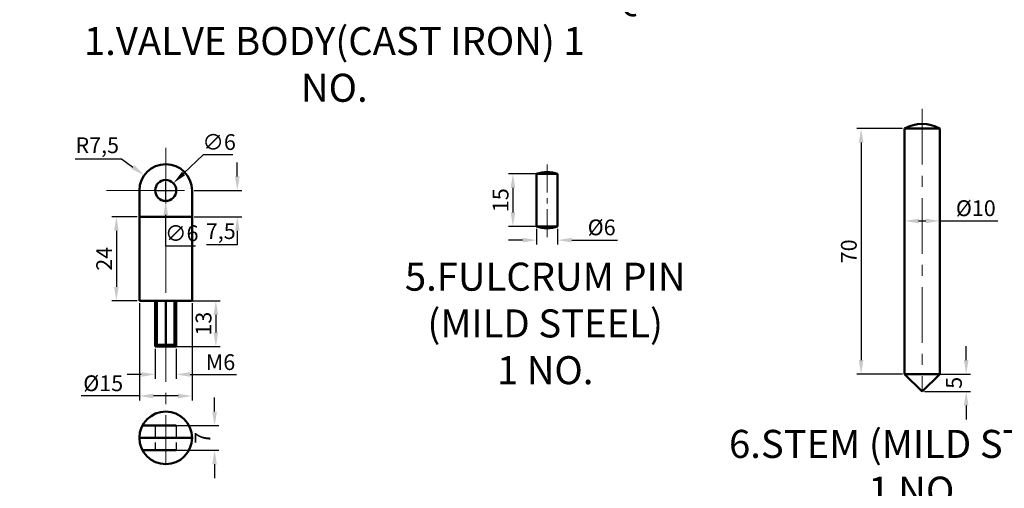
# Model space of a CAD drawing. Units: millimetres. Extents: x -166 to 681, y -4360 to 126.
# Tile 3 of 7: x -22 to 259, y -213 to -80. Entities that reach past the tile are written whole.
import ezdxf
from ezdxf import colors
from ezdxf.entities.mleader import LeaderData, LeaderLine
from ezdxf.math import Vec2, Vec3

# ---------------------------------------------------------------- set-up
doc = ezdxf.new("R2010")
doc.units = ezdxf.units.MM
doc.header["$LTSCALE"] = 0.5
doc.linetypes.add('CENTER', pattern=[50.8, 31.75, -6.35, 6.35, -6.35])
doc.linetypes.add('HIDDEN', pattern=[9.525, 6.35, -3.175])
for name, color, linetype, lineweight in [('M-CNTR', 1, 'CENTER', 18), ('M-DIMS', 2, 'Continuous', 25), ('M-HIDN', 3, 'HIDDEN', 25), ('M-OUTL', 7, 'Continuous', 50), ('M-TEXT', 7, 'Continuous', 25)]:
    doc.layers.add(name, color=color, linetype=linetype, lineweight=lineweight)
doc.styles.get("Standard").update_dxf_attribs({"font": 'arial.ttf'})
doc.dimstyles.new('ISO-25', dxfattribs={"dimtxt": 4.5, "dimasz": 4, "dimexe": 1.25, "dimexo": 0.625, "dimtad": 1, "dimtoh": 1, "dimdec": 1, "dimtxsty": 'Standard', "dimcen": 2.5, "dimadec": 0, "dimazin": 0, "dimtfac": 1, "dimtdec": 1, "dimtofl": 0, "dimtmove": 0, "dimatfit": 3, "dimfxl": 1, "dimarcsym": 0})

# ---------------------------------------------------------------- blocks, each defined once
blk = doc.blocks.new('*D37')
at = {"layer": 'Defpoints', "color": 0, "ltscale": 0.5, "transparency": 16777216}
for p in [(230.7, -110.75), (218.29, -180.75), (230.7, -180.75)]:
    blk.add_point(p, dxfattribs=at)
at = {"layer": 'M-DIMS', "color": 0, "lineweight": -2, "ltscale": 0.5, "transparency": 16777216}
for p, q in [((230.08, -110.75), (217.04, -110.75)), ((218.29, -114.75), (218.29, -176.75)), ((230.08, -180.75), (217.04, -180.75))]:
    blk.add_line(p, q, dxfattribs=at)
at = {"layer": 'M-DIMS', "color": 0, "ltscale": 0.5, "transparency": 16777216}
for points in [[(217.63, -114.75), (218.96, -114.75), (218.29, -110.75)], [(217.63, -176.75), (218.96, -176.75), (218.29, -180.75)]]:
    blk.add_solid(points, dxfattribs=at)
at = {"layer": 'M-DIMS', "color": 0, "ltscale": 0.5, "transparency": 16777216, "insert": (215.37, -145.75), "char_height": 4.5, "attachment_point": 5, "rotation": 90}
blk.add_mtext('70', dxfattribs=at)
blk = doc.blocks.new('*D38')
at = {"layer": 'Defpoints', "color": 0, "ltscale": 0.5, "transparency": 16777216}
for p in [(230.7, -136.28), (240.7, -136.28), (240.7, -137.08)]:
    blk.add_point(p, dxfattribs=at)
at = {"layer": 'M-DIMS', "color": 0, "lineweight": -2, "ltscale": 0.5, "transparency": 16777216}
for p, q in [((230.7, -136.91), (230.7, -138.33)), ((234.7, -137.08), (236.7, -137.08)), ((240.7, -136.91), (240.7, -138.33)), ((240.7, -137.08), (257.28, -137.08))]:
    blk.add_line(p, q, dxfattribs=at)
at = {"layer": 'M-DIMS', "color": 0, "ltscale": 0.5, "transparency": 16777216}
for points in [[(234.7, -136.41), (234.7, -137.75), (230.7, -137.08)], [(236.7, -136.41), (236.7, -137.75), (240.7, -137.08)]]:
    blk.add_solid(points, dxfattribs=at)
at = {"layer": 'M-DIMS', "color": 0, "ltscale": 0.5, "transparency": 16777216, "insert": (250.99, -134.03), "char_height": 4.5, "attachment_point": 5}
blk.add_mtext('%%C10', dxfattribs=at)
blk = doc.blocks.new('*D39')
at = {"layer": 'Defpoints', "color": 0, "ltscale": 0.5, "transparency": 16777216}
for p in [(235.7, -180.75), (235.7, -185.75), (248.25, -185.75)]:
    blk.add_point(p, dxfattribs=at)
at = {"layer": 'M-DIMS', "color": 0, "lineweight": -2, "ltscale": 0.5, "transparency": 16777216}
for p, q in [((248.25, -176.75), (248.25, -172.75)), ((236.33, -180.75), (249.5, -180.75)), ((236.33, -185.75), (249.5, -185.75)), ((248.25, -189.75), (248.25, -193.75))]:
    blk.add_line(p, q, dxfattribs=at)
at = {"layer": 'M-DIMS', "color": 0, "ltscale": 0.5, "transparency": 16777216}
for points in [[(247.58, -176.75), (248.91, -176.75), (248.25, -180.75)], [(247.58, -189.75), (248.91, -189.75), (248.25, -185.75)]]:
    blk.add_solid(points, dxfattribs=at)
at = {"layer": 'M-DIMS', "color": 0, "ltscale": 0.5, "transparency": 16777216, "insert": (245.33, -183.25), "char_height": 4.5, "attachment_point": 5, "rotation": 90}
blk.add_mtext('5', dxfattribs=at)
blk = doc.blocks.new('*D40')
at = {"layer": 'Defpoints', "color": 0, "ltscale": 0.5, "transparency": 16777216}
for p in [(27.57, -128.38), (27.57, -135.88), (40.47, -135.88)]:
    blk.add_point(p, dxfattribs=at)
at = {"layer": 'M-DIMS', "color": 0, "lineweight": -2, "ltscale": 0.5, "transparency": 16777216}
for p, q in [((40.47, -124.38), (40.47, -120.38)), ((28.19, -128.38), (41.72, -128.38)), ((28.19, -135.88), (41.72, -135.88)), ((40.47, -139.88), (40.47, -143.88)), ((40.47, -143.88), (31.66, -143.88))]:
    blk.add_line(p, q, dxfattribs=at)
at = {"layer": 'M-DIMS', "color": 0, "ltscale": 0.5, "transparency": 16777216}
for points in [[(39.81, -124.38), (41.14, -124.38), (40.47, -128.38)], [(39.81, -139.88), (41.14, -139.88), (40.47, -135.88)]]:
    blk.add_solid(points, dxfattribs=at)
at = {"layer": 'M-DIMS', "color": 0, "ltscale": 0.5, "transparency": 16777216, "insert": (35.75, -140.56), "char_height": 4.5, "attachment_point": 5}
blk.add_mtext('7,5', dxfattribs=at)
blk = doc.blocks.new('*D41')
at = {"layer": 'Defpoints', "color": 0, "ltscale": 0.5, "transparency": 16777216}
for p in [(12.57, -135.88), (5.99, -159.88), (12.57, -159.88)]:
    blk.add_point(p, dxfattribs=at)
at = {"layer": 'M-DIMS', "color": 0, "lineweight": -2, "ltscale": 0.5, "transparency": 16777216}
for p, q in [((11.94, -135.88), (4.74, -135.88)), ((5.99, -139.88), (5.99, -155.88)), ((11.94, -159.88), (4.74, -159.88))]:
    blk.add_line(p, q, dxfattribs=at)
at = {"layer": 'M-DIMS', "color": 0, "ltscale": 0.5, "transparency": 16777216}
for points in [[(5.33, -139.88), (6.66, -139.88), (5.99, -135.88)], [(5.33, -155.88), (6.66, -155.88), (5.99, -159.88)]]:
    blk.add_solid(points, dxfattribs=at)
at = {"layer": 'M-DIMS', "color": 0, "ltscale": 0.5, "transparency": 16777216, "insert": (3.11, -147.88), "char_height": 4.5, "attachment_point": 5, "rotation": 90}
blk.add_mtext('24', dxfattribs=at)
blk = doc.blocks.new('*D42')
at = {"layer": 'Defpoints', "color": 0, "ltscale": 0.5, "transparency": 16777216}
for p in [(20.07, -159.88), (20.07, -172.88), (34.36, -172.88)]:
    blk.add_point(p, dxfattribs=at)
at = {"layer": 'M-DIMS', "color": 0, "lineweight": -2, "ltscale": 0.5, "transparency": 16777216}
for p, q in [((20.69, -159.88), (35.61, -159.88)), ((34.36, -163.88), (34.36, -168.88)), ((20.69, -172.88), (35.61, -172.88))]:
    blk.add_line(p, q, dxfattribs=at)
at = {"layer": 'M-DIMS', "color": 0, "ltscale": 0.5, "transparency": 16777216}
for points in [[(33.69, -163.88), (35.03, -163.88), (34.36, -159.88)], [(33.69, -168.88), (35.03, -168.88), (34.36, -172.88)]]:
    blk.add_solid(points, dxfattribs=at)
at = {"layer": 'M-DIMS', "color": 0, "ltscale": 0.5, "transparency": 16777216, "insert": (31.43, -166.38), "char_height": 4.5, "attachment_point": 5, "rotation": 90}
blk.add_mtext('13', dxfattribs=at)
blk = doc.blocks.new('*D43')
at = {"layer": 'Defpoints', "color": 0, "ltscale": 0.5, "transparency": 16777216}
for p in [(17.07, -172.88), (23.07, -172.88), (23.07, -180.87)]:
    blk.add_point(p, dxfattribs=at)
at = {"layer": 'M-DIMS', "color": 0, "lineweight": -2, "ltscale": 0.5, "transparency": 16777216}
for p, q in [((17.07, -173.51), (17.07, -182.12)), ((23.07, -173.51), (23.07, -182.12)), ((13.07, -180.87), (9.07, -180.87)), ((27.07, -180.87), (40.29, -180.87))]:
    blk.add_line(p, q, dxfattribs=at)
at = {"layer": 'M-DIMS', "color": 0, "ltscale": 0.5, "transparency": 16777216}
for points in [[(13.07, -180.2), (13.07, -181.53), (17.07, -180.87)], [(27.07, -180.2), (27.07, -181.53), (23.07, -180.87)]]:
    blk.add_solid(points, dxfattribs=at)
at = {"layer": 'M-DIMS', "color": 0, "ltscale": 0.5, "transparency": 16777216, "insert": (35.68, -177.94), "char_height": 4.5, "attachment_point": 5}
blk.add_mtext('M6', dxfattribs=at)
blk = doc.blocks.new('*D44')
at = {"layer": 'Defpoints', "color": 0, "ltscale": 0.5, "transparency": 16777216}
for p in [(12.57, -159.88), (27.57, -159.88), (27.57, -187.01)]:
    blk.add_point(p, dxfattribs=at)
at = {"layer": 'M-DIMS', "color": 0, "lineweight": -2, "ltscale": 0.5, "transparency": 16777216}
for p, q in [((12.57, -160.51), (12.57, -188.26)), ((27.57, -160.51), (27.57, -188.26)), ((12.57, -187.01), (-4.06, -187.01)), ((23.57, -187.01), (16.57, -187.01))]:
    blk.add_line(p, q, dxfattribs=at)
at = {"layer": 'M-DIMS', "color": 0, "ltscale": 0.5, "transparency": 16777216}
for points in [[(16.57, -186.34), (16.57, -187.68), (12.57, -187.01)], [(23.57, -186.34), (23.57, -187.68), (27.57, -187.01)]]:
    blk.add_solid(points, dxfattribs=at)
at = {"layer": 'M-DIMS', "color": 0, "ltscale": 0.5, "transparency": 16777216, "insert": (2.25, -183.96), "char_height": 4.5, "attachment_point": 5}
blk.add_mtext('%%C15', dxfattribs=at)
blk = doc.blocks.new('*D45')
at = {"layer": 'Defpoints', "color": 0, "ltscale": 0.5, "transparency": 16777216}
for p in [(13.96, -124.03), (20.07, -128.38)]:
    blk.add_point(p, dxfattribs=at)
at = {"layer": 'M-DIMS', "color": 0, "lineweight": -2, "ltscale": 0.5, "transparency": 16777216}
for p, q in [((-5.72, -119.39), (7.44, -119.39)), ((7.44, -119.39), (10.7, -121.71)), ((20.07, -130.88), (20.07, -125.88)), ((17.57, -128.38), (22.57, -128.38))]:
    blk.add_line(p, q, dxfattribs=at)
at = {"layer": 'M-DIMS', "color": 0, "ltscale": 0.5, "transparency": 16777216}
blk.add_solid([(11.09, -121.17), (10.31, -122.25), (13.96, -124.03)], dxfattribs=at)
at = {"layer": 'M-DIMS', "color": 0, "ltscale": 0.5, "transparency": 16777216, "insert": (0.55, -116.07), "char_height": 4.5, "attachment_point": 5}
blk.add_mtext('R7,5', dxfattribs=at)
blk = doc.blocks.new('*D46')
at = {"layer": 'Defpoints', "color": 0, "ltscale": 0.5, "transparency": 16777216}
for p in [(22.24, -126.31), (17.89, -130.45)]:
    blk.add_point(p, dxfattribs=at)
at = {"layer": 'M-DIMS', "color": 0, "lineweight": -2, "ltscale": 0.5, "transparency": 16777216}
for p, q in [((30.75, -118.21), (25.13, -123.56)), ((39.21, -118.21), (30.75, -118.21)), ((20.07, -130.88), (20.07, -125.88)), ((17.57, -128.38), (22.57, -128.38))]:
    blk.add_line(p, q, dxfattribs=at)
at = {"layer": 'M-DIMS', "color": 0, "ltscale": 0.5, "transparency": 16777216}
blk.add_solid([(24.68, -123.07), (25.59, -124.04), (22.24, -126.31)], dxfattribs=at)
at = {"layer": 'M-DIMS', "color": 0, "ltscale": 0.5, "transparency": 16777216, "insert": (35.29, -115.16), "char_height": 4.5, "attachment_point": 5}
blk.add_mtext('∅6', dxfattribs=at)
blk = doc.blocks.new('*D47')
at = {"layer": 'Defpoints', "color": 0, "ltscale": 0.5, "transparency": 16777216}
for p in [(20.07, -195.46), (18.25, -202.46), (34, -202.46)]:
    blk.add_point(p, dxfattribs=at)
at = {"layer": 'M-DIMS', "color": 0, "lineweight": -2, "ltscale": 0.5, "transparency": 16777216}
for p, q in [((34, -191.46), (34, -187.46)), ((20.69, -195.46), (35.25, -195.46)), ((18.87, -202.46), (35.25, -202.46)), ((34, -206.46), (34, -210.46))]:
    blk.add_line(p, q, dxfattribs=at)
at = {"layer": 'M-DIMS', "color": 0, "ltscale": 0.5, "transparency": 16777216}
for points in [[(33.33, -191.46), (34.67, -191.46), (34, -195.46)], [(33.33, -206.46), (34.67, -206.46), (34, -202.46)]]:
    blk.add_solid(points, dxfattribs=at)
at = {"layer": 'M-DIMS', "color": 0, "ltscale": 0.5, "transparency": 16777216, "insert": (31.13, -198.96), "char_height": 4.5, "attachment_point": 5, "rotation": 90}
blk.add_mtext('7', dxfattribs=at)
blk = doc.blocks.new('*D53')
at = {"layer": 'Defpoints', "color": 0, "ltscale": 0.5, "transparency": 16777216}
for p in [(125.79, -138.66), (131.79, -138.66), (131.79, -142.55)]:
    blk.add_point(p, dxfattribs=at)
at = {"layer": 'M-DIMS', "color": 0, "lineweight": -2, "ltscale": 0.5, "transparency": 16777216}
for p, q in [((125.79, -139.29), (125.79, -143.8)), ((131.79, -139.29), (131.79, -143.8)), ((121.79, -142.55), (117.79, -142.55)), ((135.79, -142.55), (148.88, -142.55))]:
    blk.add_line(p, q, dxfattribs=at)
at = {"layer": 'M-DIMS', "color": 0, "ltscale": 0.5, "transparency": 16777216}
for points in [[(121.79, -141.88), (121.79, -143.21), (125.79, -142.55)], [(135.79, -141.88), (135.79, -143.21), (131.79, -142.55)]]:
    blk.add_solid(points, dxfattribs=at)
at = {"layer": 'M-DIMS', "color": 0, "ltscale": 0.5, "transparency": 16777216, "insert": (144.34, -139.5), "char_height": 4.5, "attachment_point": 5}
blk.add_mtext('%%C6', dxfattribs=at)
blk = doc.blocks.new('*D54')
at = {"layer": 'Defpoints', "color": 0, "ltscale": 0.5, "transparency": 16777216}
for p in [(128.79, -123.66), (119.03, -138.66), (128.79, -138.66)]:
    blk.add_point(p, dxfattribs=at)
at = {"layer": 'M-DIMS', "color": 0, "lineweight": -2, "ltscale": 0.5, "transparency": 16777216}
for p, q in [((128.17, -123.66), (117.78, -123.66)), ((119.03, -127.66), (119.03, -134.66)), ((128.17, -138.66), (117.78, -138.66))]:
    blk.add_line(p, q, dxfattribs=at)
at = {"layer": 'M-DIMS', "color": 0, "ltscale": 0.5, "transparency": 16777216}
for points in [[(118.37, -127.66), (119.7, -127.66), (119.03, -123.66)], [(118.37, -134.66), (119.7, -134.66), (119.03, -138.66)]]:
    blk.add_solid(points, dxfattribs=at)
at = {"layer": 'M-DIMS', "color": 0, "ltscale": 0.5, "transparency": 16777216, "insert": (116.11, -131.16), "char_height": 4.5, "attachment_point": 5, "rotation": 90}
blk.add_mtext('15', dxfattribs=at)
blk = doc.blocks.new('*D103')
at = {"layer": 'Defpoints', "color": 0, "ltscale": 0.5, "transparency": 16777216}
for p in [(20.06, -125.38), (20.07, -131.38)]:
    blk.add_point(p, dxfattribs=at)
at = {"layer": 'M-DIMS', "color": 0, "lineweight": -2, "ltscale": 0.5, "transparency": 16777216}
for p, q in [((20.07, -130.88), (20.07, -125.88)), ((17.57, -128.38), (22.57, -128.38)), ((20.08, -144.23), (20.07, -135.38)), ((28.55, -144.23), (20.08, -144.23))]:
    blk.add_line(p, q, dxfattribs=at)
at = {"layer": 'M-DIMS', "color": 0, "ltscale": 0.5, "transparency": 16777216}
blk.add_solid([(20.74, -135.38), (19.41, -135.38), (20.07, -131.38)], dxfattribs=at)
at = {"layer": 'M-DIMS', "color": 0, "ltscale": 0.5, "transparency": 16777216, "insert": (24.63, -141.18), "char_height": 4.5, "attachment_point": 5}
blk.add_mtext('∅6', dxfattribs=at)

msp = doc.modelspace()

# ---------------------------------------------------------------- linework, layer by layer
at = {"layer": 'M-CNTR'}
for p, q in [((235.7045, -105.1403), (235.7045, -185.7528)), ((20.0667, -116.2736), (20.0667, -206.459)), ((3.1676, -128.3839), (35.5663, -128.3839))]:
    msp.add_line(p, q, dxfattribs=at)
at = {"layer": 'M-CNTR', "ltscale": 0.5}
msp.add_line((128.7913, -121.025), (128.7913, -142.5717), dxfattribs=at)
at = {"layer": 'M-HIDN'}
for p, q in [((17.0667, -195.4642), (17.0667, -202.4565)), ((23.0667, -195.463), (23.0667, -202.4565))]:
    msp.add_line(p, q, dxfattribs=at)
at = {"layer": 'M-OUTL'}
for p, q in [((230.7045, -110.7528), (230.7045, -180.7528)), ((240.7045, -110.7528), (230.7045, -110.7528)), ((240.7045, -180.7528), (240.7045, -110.7528)), ((12.5667, -128.3839), (12.5667, -159.8839)), ((27.5667, -128.3839), (27.5667, -159.8839)), ((12.5667, -135.8839), (27.5667, -135.8839)), ((12.5667, -159.8839), (27.5667, -159.8839)), ((17.0667, -159.8839), (17.0667, -172.8839)), ((17.5667, -159.8839), (17.5667, -172.8839)), ((20.0667, -159.8839), (20.0667, -172.8839)), ((22.5667, -159.8839), (22.5667, -172.8839)), ((23.0667, -159.8839), (23.0667, -172.8839)), ((17.0667, -172.3839), (23.0667, -172.3839)), ((17.5667, -172.8839), (17.0667, -172.3839)), ((17.0667, -172.8839), (23.0667, -172.8839)), ((22.5667, -172.8839), (23.0667, -172.3839)), ((230.7045, -180.7528), (240.7045, -180.7528)), ((235.7045, -185.7528), (230.7045, -180.7528)), ((235.7045, -185.7528), (240.7045, -180.7528)), ((23.0667, -195.4642), (13.4307, -195.4642)), ((27.5667, -198.959), (12.5667, -198.959)), ((23.0667, -202.4565), (13.4322, -202.4565))]:
    msp.add_line(p, q, dxfattribs=at)
at = {"layer": 'M-OUTL', "ltscale": 0.5}
for p, q in [((125.7913, -123.6625), (125.7913, -138.6625)), ((131.7913, -123.6625), (125.7913, -123.6625)), ((131.7913, -138.6625), (131.7913, -123.6625)), ((125.7913, -138.6625), (131.7913, -138.6625))]:
    msp.add_line(p, q, dxfattribs=at)
at = {"layer": 'M-OUTL'}
for centre, radius in [((20.0667, -128.3839), 3), ((20.0667, -198.959), 7.5)]:
    msp.add_circle(centre, radius, dxfattribs=at)
for centre, radius, start, end in [((235.7045, -119.4131), 10, 60, 120), ((20.0667, -128.3839), 7.5, 0, 180)]:
    msp.add_arc(centre, radius, start, end, dxfattribs=at)
at = {"layer": 'M-OUTL', "ltscale": 0.5}
for centre, radius, start, end in [((128.7913, -132.3272), 9.1694, 70.902483, 109.097517), ((128.7913, -130.691), 8.5174, 249.376778, 290.623222)]:
    msp.add_arc(centre, radius, start, end, dxfattribs=at)

# ---------------------------------------------------------------- texts
at = {"layer": 'M-TEXT', "ltscale": 0.5, "char_height": 8, "attachment_point": 1}
for s, insert in [('\\pxqc;1.VALVE BODY(CAST IRON) 1 NO.', (-7.3401, -81.7631)), ('\\pxqc;5.FULCRUM PIN\\P(MILD STEEL) \\P1 NO.', (52.7666, -148.975)), ('\\pxqc;6.STEM (MILD STEEL) \\P1 NO.', (158.6774, -196.6773))]:
    msp.add_mtext_dynamic_manual_height_columns(s, width=150.92987, gutter_width=12.5, heights=[0], dxfattribs=dict(at, insert=insert))

# ---------------------------------------------------------------- dimensions: what is measured, and where the dimension line sits
at = {"layer": 'M-DIMS', "ltscale": 0.5}
for p1, p2, override, picture, middle in [((17.8947, -130.4532), (22.2388, -126.3146), {"dimclrd": 0, "dimclre": 0, "dimclrt": 0}, '*D46', (35.2916, -118.2106)), ((20.0635, -125.3839), (20.07, -131.3839), {"dimdec": 0, "dimlfac": 1, "dimrnd": 0, "dimzin": 0, "dimdsep": 46, "dimlunit": 2}, '*D103', (24.6304, -144.2308))]:
    dim = msp.add_diameter_dim_2p(p1=p1, p2=p2, dimstyle='ISO-25', override=override, dxfattribs=at)
    dim.commit()
    dim.dimension.update_dxf_attribs({"geometry": picture, "text_midpoint": middle, "dimtype": 163})
for base, p1, p2, picture, middle in [((218.2945, -180.7528), (230.7045, -110.7528), (230.7045, -180.7528), '*D37', (215.3719, -145.7528)), ((40.4735, -135.8839), (27.5667, -128.3839), (27.5667, -135.8839), '*D40', (35.7537, -140.5638)), ((119.0332, -138.6625), (128.7913, -123.6625), (128.7913, -138.6625), '*D54', (116.1106, -131.1625)), ((5.9944, -159.8839), (12.5667, -135.8839), (12.5667, -159.8839), '*D41', (3.1102, -147.8839)), ((34.3589, -172.8839), (20.0667, -159.8839), (20.0667, -172.8839), '*D42', (31.4348, -166.3839)), ((248.2464, -185.7528), (235.7045, -180.7528), (235.7045, -185.7528), '*D39', (245.333, -183.2528)), ((34.0016, -202.4565), (20.0667, -195.463), (18.2495, -202.4565), '*D47', (31.1266, -198.9597))]:
    dim = msp.add_linear_dim(base=base, p1=p1, p2=p2, angle=90, dimstyle='ISO-25', override={"dimclrd": 0, "dimclre": 0, "dimclrt": 0}, dxfattribs=at)
    dim.commit()
    dim.dimension.update_dxf_attribs({"geometry": picture, "text_midpoint": middle})
dim = msp.add_radius_dim(center=(20.0667, -128.3839), mpoint=(13.9581, -124.0325), dimstyle='ISO-25', override={"dimclrd": 0, "dimclre": 0, "dimclrt": 0}, dxfattribs=at)
dim.commit()
dim.dimension.update_dxf_attribs({"geometry": '*D45', "text_midpoint": (0.5507, -116.0709)})
dim = msp.add_linear_dim(base=(240.7045, -137.0786), p1=(230.7045, -136.28), p2=(240.7045, -136.28), text='%%C<>', dimstyle='ISO-25', override={"dimclrd": 0, "dimclre": 0, "dimclrt": 0}, dxfattribs=at)
dim.commit()
dim.dimension.update_dxf_attribs({"geometry": '*D38', "text_midpoint": (250.9929, -134.0302)})
for base, p1, p2, text, picture, middle in [((131.7913, -142.5456), (125.7913, -138.6625), (131.7913, -138.6625), '%%C<>', '*D53', (144.3377, -142.5456)), ((27.5667, -187.0086), (12.5667, -159.8839), (27.5667, -159.8839), '%%C<>', '*D44', (2.2538, -187.0086)), ((23.0667, -180.8663), (17.0667, -172.8839), (23.0667, -172.8839), 'M<>', '*D43', (35.6806, -180.8663))]:
    dim = msp.add_linear_dim(base=base, p1=p1, p2=p2, text=text, dimstyle='ISO-25', override={"dimclrd": 0, "dimclre": 0, "dimclrt": 0}, dxfattribs=at)
    dim.commit()
    dim.dimension.update_dxf_attribs({"geometry": picture, "text_midpoint": middle, "dimtype": 160})

# ---------------------------------------------------------------- leaders
at = {"layer": 'M-TEXT', "ltscale": 0.5}
ml = msp.add_multileader_mtext('Standard', dxfattribs=at)
ml.set_content('4 HOLES DIA 8,\\P EQI SP  PCD 56', color=256)
ml.set_leader_properties()
ml.build(insert=Vec2(0, 0))
ctx = ml.context
ctx.base_point, ctx.char_height, ctx.plane_origin = Vec3(-78.2306, -49.2827), 7, Vec3(28.8008, -13.8088)
ctx.text_align_type = 2
notes = []
notes.append((ctx, [(0, (1, 1, 0), (8.3199, -49.2827), (-1, 0), 8, [(0, [(28.8008, -13.8088)], 0, [])])]))
ctx.mtext.insert, ctx.mtext.alignment, ctx.mtext.flow_direction = Vec3(-1.6801, -45.5106), 3, 5
ml = msp.add_multileader_mtext('Standard', dxfattribs=at)
ml.set_content('4 HOLES DIA 8,\\P EQI SP  PCD 56', color=256)
ml.set_leader_properties()
ml.build(insert=Vec2(0, 0))
ctx = ml.context
ctx.base_point, ctx.char_height, ctx.plane_origin = Vec3(139.9432, -62.1565), 7, Vec3(114.3904, -39.5588)
notes.append((ctx, [(1, (1, 1, 0), (131.9432, -62.1565), (1, 0), 8, [(0, [(114.3904, -39.5588)], 0, [])])]))
ctx.mtext.insert, ctx.mtext.flow_direction = Vec3(141.9432, -58.3843), 5
for ctx, leaders in notes:
    for number, flags, end, landing, length, lines in leaders:
        leader = LeaderData()
        leader.index, (leader.has_last_leader_line, leader.has_dogleg_vector, leader.attachment_direction) = number, flags
        leader.last_leader_point, leader.dogleg_vector, leader.dogleg_length = Vec3(end), Vec3(landing), length
        for number, points, colour, breaks in lines:
            line = LeaderLine()
            line.index, line.vertices, line.color, line.breaks = number, Vec3.list(points), colors.encode_raw_color(colour), breaks
            leader.lines.append(line)
        ctx.leaders.append(leader)

doc.saveas('drawing.dxf')
